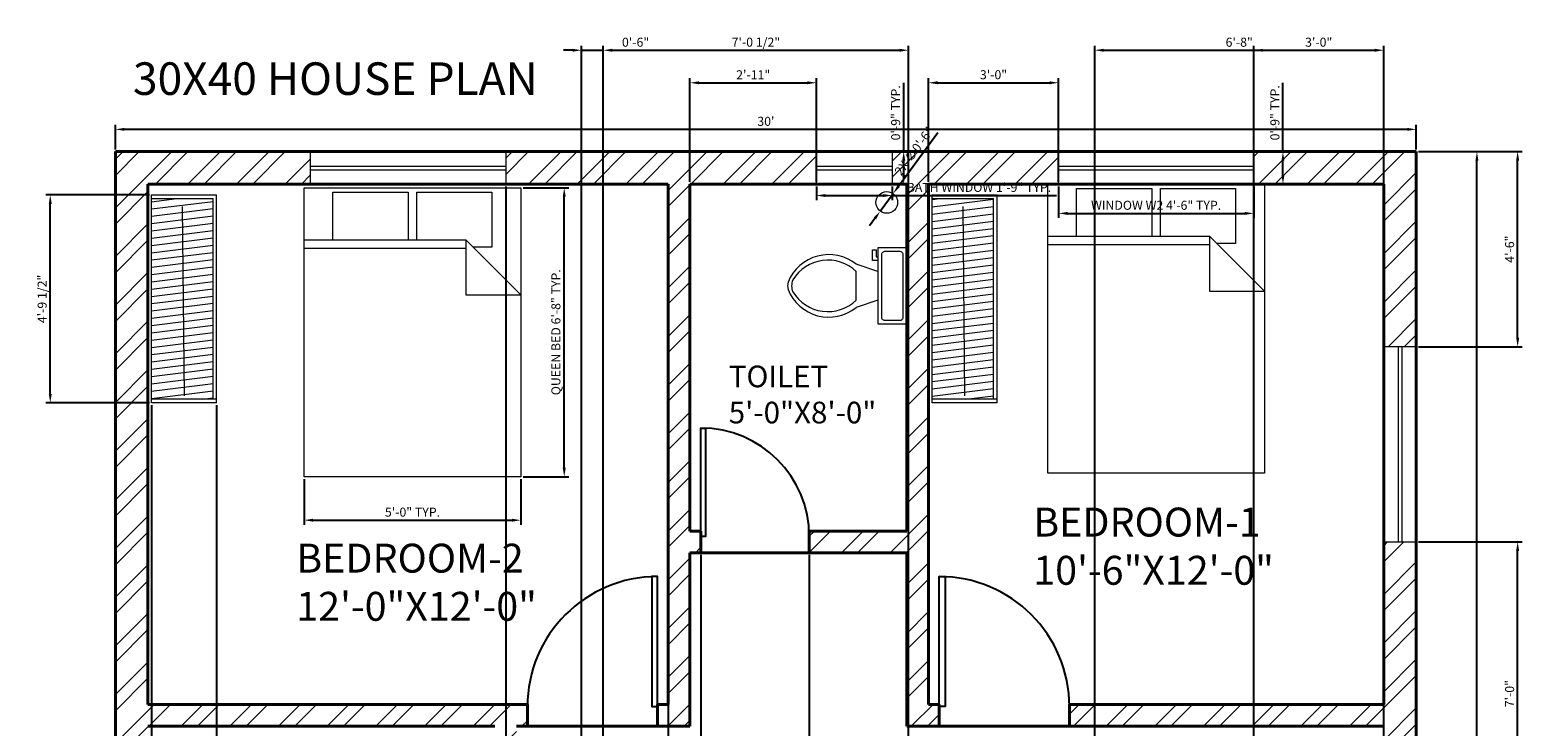
# Model space of a CAD drawing. Units: inches. Extents: x 201 to 622, y 55 to 632.
# Tile 3 of 3: x 209 to 622, y 439 to 632. Entities that reach past the tile are written whole.
import ezdxf

# ---------------------------------------------------------------- set-up
doc = ezdxf.new("R2010")
doc.units = ezdxf.units.IN
for name, color, linetype, lineweight in [('A-ANNO-DIMS', 2, 'Continuous', 18), ('A-ANNO-TITL', 7, 'Continuous', 25), ('A-AREA-IDEN', 7, 'Continuous', 18), ('A-DOOR', 4, 'Continuous', 25), ('A-FLOR-CASE', 8, 'Continuous', 18), ('A-FLOR-CASE-PATT', 8, 'Continuous', 13), ('A-FLOR-FIXT', 8, 'Continuous', 18), ('A-WALL', 7, 'Continuous', 40), ('A-WALL-PATT', 252, 'Continuous', 13)]:
    doc.layers.add(name, color=color, linetype=linetype, lineweight=lineweight)
doc.layers.add('A-FURN', color=152, linetype='Continuous', lineweight=18, true_color=0x2776bb)
doc.layers.add('A-GLAZ', color=152, linetype='Continuous', lineweight=18, true_color=0x2776bb)
doc.styles.get("Standard").update_dxf_attribs({"font": 'arial.ttf'})
doc.dimstyles.new('ISO-25', dxfattribs={"dimtxt": 2.5, "dimasz": 2.5, "dimexe": 1.25, "dimexo": 0.625, "dimtad": 1, "dimlunit": 3, "dimtxsty": 'Standard', "dimcen": 2.5, "dimadec": 0, "dimazin": 0, "dimtfac": 1, "dimtmove": 0, "dimatfit": 3, "dimfxl": 1, "dimarcsym": 0})

# ---------------------------------------------------------------- blocks, each defined once
blk = doc.blocks.new('*U2')
for p, q in [((0, 0), (0, -6)), ((-40, 0), (-40, -6))]:
    blk.add_line(p, q)
blk.add_lwpolyline([(0, 0), (0, 40), (-1.75, 40), (-1.75, 0)], close=True)
blk.add_arc((0, 0), 40, 90, 180)
blk = doc.blocks.new('*U3')
for p, q in [((0, 0), (0, -6)), ((40, 0), (40, -6))]:
    blk.add_line(p, q)
blk.add_lwpolyline([(0, 0), (0, 40), (1.75, 40), (1.75, 0)], close=True)
blk.add_arc((0, 0), 40, 0, 90)
blk = doc.blocks.new('Bed - Queen')
for p, q in [((0, -80.00003), (0, 0)), ((0, 0), (59.99999, 0)), ((59.99999, 0), (59.99999, -80.00003)), ((7.99999, -1.2), (28.79998, -1.2)), ((7.99999, -14.4), (7.99999, -1.2)), ((28.79998, -1.2), (28.79998, -14.4)), ((31.19999, -1.2), (51.99999, -1.2)), ((31.19999, -14.4), (31.19999, -1.2)), ((51.99999, -1.2), (51.99999, -16.4)), ((0, -14.4), (44.8, -14.4)), ((59.99999, -29.6), (44.8, -14.4)), ((44.8, -14.4), (44.8, -29.6)), ((51.99999, -16.4), (46.79936, -16.4)), ((44.8, -16.8), (0, -16.8)), ((44.8, -29.6), (59.99999, -29.6)), ((59.99999, -80.00003), (0, -80.00003))]:
    blk.add_line(p, q)
blk = doc.blocks.new('*U9')
for p, q in [((9.5, -6), (9.5, -2)), ((-8, -8.5), (-8, -8)), ((-7, -8), (-7, -9.5)), ((-4, -8), (-6, -14)), ((4, -8), (6, -14)), ((-10, -8.5), (-8, -8.5)), ((-10, -9.5), (-10, -8.5)), ((-7, -9.5), (-10, -9.5)), ((4, -14), (-4, -14))]:
    blk.add_line(p, q)
blk.add_lwpolyline([(10.5, -8), (10.5, 0), (-10.5, 0), (-10.5, -8)], close=True)
for points in [[(-9.5, -2), (-9.5, -6)], [(8.5, -1), (-8.5, -1)], [(-8.5, -7), (8.5, -7)]]:
    blk.add_lwpolyline(points)
for centre, radius, start, end in [((-8.62, -1.88), 0.884, 81.8699, 188.1301), ((8.62, -1.88), 0.884, 351.8699, 98.1301), ((-8.62, -6.12), 0.884, 171.8699, 278.1301), ((8.62, -6.12), 0.884, 261.8699, 8.1301), ((3.52, -21.58), 12.17, 141.4691, 247.9714), ((4.2, -21.82), 11.33, 136.3677, 238.9468), ((-3.52, -21.58), 12.17, 292.0284, 38.5307), ((-4.2, -21.82), 11.33, 301.053, 43.6321), ((0, -27.88), 4, 245.7318, 294.2682), ((0, -29), 4, 254.8605, 285.1395)]:
    blk.add_arc(centre, radius, start, end)
blk = doc.blocks.new('*D10')
at = {"layer": 'A-ANNO-DIMS', "color": 0, "lineweight": -2, "transparency": 16777216}
for p, q in [((592.99, 598.15), (610.4, 598.15)), ((609.15, 120.65), (609.15, 595.65)), ((592.99, 118.15), (610.4, 118.15))]:
    blk.add_line(p, q, dxfattribs=at)
at = {"layer": 'A-ANNO-DIMS', "color": 0, "transparency": 16777216}
for points in [[(608.73, 595.65), (609.56, 595.65), (609.15, 598.15)], [(608.73, 120.65), (609.56, 120.65), (609.15, 118.15)]]:
    blk.add_solid(points, dxfattribs=at)
at = {"layer": 'Defpoints', "color": 0, "transparency": 16777216}
for p in [(592.36, 598.15), (609.15, 598.15), (592.36, 118.15)]:
    blk.add_point(p, dxfattribs=at)
at = {"layer": 'A-ANNO-DIMS', "color": 0, "transparency": 16777216, "insert": (607.25, 358.15), "char_height": 2.5, "attachment_point": 5, "rotation": 90}
blk.add_mtext("40'", dxfattribs=at)
blk = doc.blocks.new('*D11')
at = {"layer": 'A-ANNO-DIMS', "color": 0, "lineweight": -2, "transparency": 16777216}
for p, q in [((232.36, 598.77), (232.36, 605.55)), ((589.86, 604.3), (234.86, 604.3)), ((592.36, 598.77), (592.36, 605.55))]:
    blk.add_line(p, q, dxfattribs=at)
at = {"layer": 'A-ANNO-DIMS', "color": 0, "transparency": 16777216}
for points in [[(234.86, 604.72), (234.86, 603.89), (232.36, 604.3)], [(589.86, 604.72), (589.86, 603.89), (592.36, 604.3)]]:
    blk.add_solid(points, dxfattribs=at)
at = {"layer": 'Defpoints', "color": 0, "transparency": 16777216}
for p in [(232.36, 604.3), (232.36, 598.15), (592.36, 598.15)]:
    blk.add_point(p, dxfattribs=at)
at = {"layer": 'A-ANNO-DIMS', "color": 0, "transparency": 16777216, "insert": (412.36, 606.2), "char_height": 2.5, "attachment_point": 5}
blk.add_mtext("30'", dxfattribs=at)
blk = doc.blocks.new('WIN-54')
for p, q in [((0, 5), (54, 5)), ((0, 4), (54, 4))]:
    blk.add_line(p, q)
blk.add_lwpolyline([(0, 9), (54, 9), (54, 0), (0, 0)], close=True)
blk = doc.blocks.new('WIN-21')
for p, q in [((0, 5), (21, 5)), ((0, 4), (21, 4))]:
    blk.add_line(p, q)
blk.add_lwpolyline([(0, 0), (0, 9), (21, 9), (21, 0)], close=True)
blk = doc.blocks.new('WIN-54-B')
for p, q in [((0, 5), (54, 5)), ((0, 4), (54, 4))]:
    blk.add_line(p, q)
blk.add_lwpolyline([(0, 9), (54, 9), (54, 0), (0, 0)], close=True)
blk = doc.blocks.new('*D17')
at = {"layer": 'A-ANNO-DIMS', "color": 0, "lineweight": -2, "transparency": 16777216}
for p, q in [((493.36, 588.52), (493.36, 579.8)), ((547.36, 588.52), (547.36, 579.8)), ((495.86, 581.05), (544.86, 581.05))]:
    blk.add_line(p, q, dxfattribs=at)
at = {"layer": 'A-ANNO-DIMS', "color": 0, "transparency": 16777216}
for points in [[(495.86, 581.46), (495.86, 580.63), (493.36, 581.05)], [(544.86, 581.46), (544.86, 580.63), (547.36, 581.05)]]:
    blk.add_solid(points, dxfattribs=at)
at = {"layer": 'Defpoints', "color": 0, "transparency": 16777216}
for p in [(493.36, 589.15), (547.36, 589.15), (547.36, 581.05)]:
    blk.add_point(p, dxfattribs=at)
at = {"layer": 'A-ANNO-DIMS', "color": 0, "transparency": 16777216, "insert": (520.36, 582.97), "char_height": 2.5, "attachment_point": 5}
blk.add_mtext('WINDOW W2 4\'-6" TYP.', dxfattribs=at)
blk = doc.blocks.new('*D18')
at = {"layer": 'A-ANNO-DIMS', "color": 0, "lineweight": -2, "transparency": 16777216}
for p, q in [((555.46, 598.15), (555.46, 617.14)), ((547.99, 598.15), (556.71, 598.15)), ((555.46, 591.65), (555.46, 595.65)), ((547.99, 589.15), (556.71, 589.15))]:
    blk.add_line(p, q, dxfattribs=at)
at = {"layer": 'A-ANNO-DIMS', "color": 0, "transparency": 16777216}
for points in [[(555.05, 595.65), (555.88, 595.65), (555.46, 598.15)], [(555.05, 591.65), (555.88, 591.65), (555.46, 589.15)]]:
    blk.add_solid(points, dxfattribs=at)
at = {"layer": 'Defpoints', "color": 0, "transparency": 16777216}
for p in [(547.36, 598.15), (555.46, 598.15), (547.36, 589.15)]:
    blk.add_point(p, dxfattribs=at)
at = {"layer": 'A-ANNO-DIMS', "color": 0, "transparency": 16777216, "insert": (553.56, 608.89), "char_height": 2.5, "attachment_point": 5, "rotation": 90}
blk.add_mtext('0\'-9" TYP.', dxfattribs=at)
blk = doc.blocks.new('*D19')
at = {"layer": 'A-ANNO-DIMS', "color": 0, "lineweight": -2, "transparency": 16777216}
for p, q in [((426.35, 588.52), (426.35, 584.75)), ((447.35, 588.52), (447.35, 584.75)), ((428.85, 586), (444.85, 586)), ((447.35, 586), (492.81, 586))]:
    blk.add_line(p, q, dxfattribs=at)
at = {"layer": 'A-ANNO-DIMS', "color": 0, "transparency": 16777216}
for points in [[(428.85, 586.41), (428.85, 585.58), (426.35, 586)], [(444.85, 586.41), (444.85, 585.58), (447.35, 586)]]:
    blk.add_solid(points, dxfattribs=at)
at = {"layer": 'Defpoints', "color": 0, "transparency": 16777216}
for p in [(426.35, 589.15), (447.35, 589.15), (447.35, 586)]:
    blk.add_point(p, dxfattribs=at)
at = {"layer": 'A-ANNO-DIMS', "color": 0, "transparency": 16777216, "insert": (471.33, 587.92), "char_height": 2.5, "attachment_point": 5}
blk.add_mtext('BATH WINDOW 1\'-9" TYP.', dxfattribs=at)
blk = doc.blocks.new('*D20')
at = {"layer": 'A-ANNO-DIMS', "color": 0, "lineweight": -2, "transparency": 16777216}
for p, q in [((450.5, 598.15), (450.5, 617.14)), ((447.98, 598.15), (451.75, 598.15)), ((450.5, 591.65), (450.5, 595.65)), ((447.98, 589.15), (451.75, 589.15))]:
    blk.add_line(p, q, dxfattribs=at)
at = {"layer": 'A-ANNO-DIMS', "color": 0, "transparency": 16777216}
for points in [[(450.09, 595.65), (450.92, 595.65), (450.5, 598.15)], [(450.09, 591.65), (450.92, 591.65), (450.5, 589.15)]]:
    blk.add_solid(points, dxfattribs=at)
at = {"layer": 'Defpoints', "color": 0, "transparency": 16777216}
for p in [(447.35, 598.15), (450.5, 598.15), (447.35, 589.15)]:
    blk.add_point(p, dxfattribs=at)
at = {"layer": 'A-ANNO-DIMS', "color": 0, "transparency": 16777216, "insert": (448.6, 608.89), "char_height": 2.5, "attachment_point": 5, "rotation": 90}
blk.add_mtext('0\'-9" TYP.', dxfattribs=at)
blk = doc.blocks.new('*D21')
at = {"layer": 'A-ANNO-DIMS', "color": 0, "lineweight": -2, "transparency": 16777216}
for p, q in [((345.19, 588.15), (357.81, 588.15)), ((356.56, 510.65), (356.56, 585.65)), ((345.19, 508.15), (357.81, 508.15))]:
    blk.add_line(p, q, dxfattribs=at)
at = {"layer": 'A-ANNO-DIMS', "color": 0, "transparency": 16777216}
for points in [[(356.15, 585.65), (356.98, 585.65), (356.56, 588.15)], [(356.15, 510.65), (356.98, 510.65), (356.56, 508.15)]]:
    blk.add_solid(points, dxfattribs=at)
at = {"layer": 'Defpoints', "color": 0, "transparency": 16777216}
for p in [(344.56, 588.15), (356.56, 588.15), (344.56, 508.15)]:
    blk.add_point(p, dxfattribs=at)
at = {"layer": 'A-ANNO-DIMS', "color": 0, "transparency": 16777216, "insert": (354.57, 548.15), "char_height": 2.5, "attachment_point": 5, "rotation": 90}
blk.add_mtext('QUEEN BED 6\'-8" TYP.', dxfattribs=at)
blk = doc.blocks.new('*D22')
at = {"layer": 'A-ANNO-DIMS', "color": 0, "lineweight": -2, "transparency": 16777216}
for p, q in [((284.56, 507.52), (284.56, 494.9)), ((344.56, 507.52), (344.56, 494.9)), ((287.06, 496.15), (342.06, 496.15))]:
    blk.add_line(p, q, dxfattribs=at)
at = {"layer": 'A-ANNO-DIMS', "color": 0, "transparency": 16777216}
for points in [[(287.06, 496.56), (287.06, 495.73), (284.56, 496.15)], [(342.06, 496.56), (342.06, 495.73), (344.56, 496.15)]]:
    blk.add_solid(points, dxfattribs=at)
at = {"layer": 'Defpoints', "color": 0, "transparency": 16777216}
for p in [(284.56, 508.15), (344.56, 508.15), (344.56, 496.15)]:
    blk.add_point(p, dxfattribs=at)
at = {"layer": 'A-ANNO-DIMS', "color": 0, "transparency": 16777216, "insert": (314.56, 498.05), "char_height": 2.5, "attachment_point": 5}
blk.add_mtext('5\'-0" TYP.', dxfattribs=at)
blk = doc.blocks.new('*D26')
at = {"layer": 'A-ANNO-DIMS', "color": 0, "lineweight": -2, "transparency": 16777216}
for p, q in [((547.36, 319.77), (547.36, 627.45)), ((549.86, 626.2), (580.86, 626.2)), ((583.36, 319.77), (583.36, 627.45))]:
    blk.add_line(p, q, dxfattribs=at)
at = {"layer": 'A-ANNO-DIMS', "color": 0, "transparency": 16777216}
for points in [[(549.86, 626.61), (549.86, 625.78), (547.36, 626.2)], [(580.86, 626.61), (580.86, 625.78), (583.36, 626.2)]]:
    blk.add_solid(points, dxfattribs=at)
at = {"layer": 'Defpoints', "color": 0, "transparency": 16777216}
for p in [(583.36, 626.2), (547.36, 319.15), (583.36, 319.15)]:
    blk.add_point(p, dxfattribs=at)
at = {"layer": 'A-ANNO-DIMS', "color": 0, "transparency": 16777216, "insert": (565.36, 628.1), "char_height": 2.5, "attachment_point": 5}
blk.add_mtext('3\'-0"', dxfattribs=at)
blk = doc.blocks.new('*D27')
at = {"layer": 'A-ANNO-DIMS', "color": 0, "lineweight": -2, "transparency": 16777216}
for p, q in [((358.86, 626.2), (356.36, 626.2)), ((361.36, 289.77), (361.36, 627.45)), ((361.36, 626.2), (367.36, 626.2)), ((367.36, 289.77), (367.36, 627.45)), ((369.86, 626.2), (380.26, 626.2))]:
    blk.add_line(p, q, dxfattribs=at)
at = {"layer": 'A-ANNO-DIMS', "color": 0, "transparency": 16777216}
for points in [[(358.86, 626.61), (358.86, 625.78), (361.36, 626.2)], [(369.86, 626.61), (369.86, 625.78), (367.36, 626.2)]]:
    blk.add_solid(points, dxfattribs=at)
at = {"layer": 'Defpoints', "color": 0, "transparency": 16777216}
for p in [(367.36, 626.2), (361.36, 289.15), (367.36, 289.15)]:
    blk.add_point(p, dxfattribs=at)
at = {"layer": 'A-ANNO-DIMS', "color": 0, "transparency": 16777216, "insert": (376.31, 628.1), "char_height": 2.5, "attachment_point": 5}
blk.add_mtext('0\'-6"', dxfattribs=at)
blk = doc.blocks.new('*D29')
at = {"layer": 'A-ANNO-DIMS', "color": 0, "lineweight": -2, "transparency": 16777216}
for p, q in [((340.36, 588.52), (340.36, 55.85)), ((385.36, 588.52), (385.36, 55.85)), ((342.86, 57.1), (382.86, 57.1))]:
    blk.add_line(p, q, dxfattribs=at)
at = {"layer": 'A-ANNO-DIMS', "color": 0, "transparency": 16777216}
for points in [[(342.86, 57.51), (342.86, 56.68), (340.36, 57.1)], [(382.86, 57.51), (382.86, 56.68), (385.36, 57.1)]]:
    blk.add_solid(points, dxfattribs=at)
at = {"layer": 'Defpoints', "color": 0, "transparency": 16777216}
for p in [(340.36, 589.15), (385.36, 589.15), (385.36, 57.1)]:
    blk.add_point(p, dxfattribs=at)
at = {"layer": 'A-ANNO-DIMS', "color": 0, "transparency": 16777216, "insert": (362.86, 59), "char_height": 2.5, "attachment_point": 5}
blk.add_mtext('3\'-9"', dxfattribs=at)
blk = doc.blocks.new('*D30')
at = {"layer": 'A-ANNO-DIMS', "color": 0, "lineweight": -2, "transparency": 16777216}
for p, q in [((391.36, 589.77), (391.36, 618.45)), ((393.86, 617.2), (423.85, 617.2)), ((426.35, 589.77), (426.35, 618.45))]:
    blk.add_line(p, q, dxfattribs=at)
at = {"layer": 'A-ANNO-DIMS', "color": 0, "transparency": 16777216}
for points in [[(393.86, 617.61), (393.86, 616.78), (391.36, 617.2)], [(423.85, 617.61), (423.85, 616.78), (426.35, 617.2)]]:
    blk.add_solid(points, dxfattribs=at)
at = {"layer": 'Defpoints', "color": 0, "transparency": 16777216}
for p in [(426.35, 617.2), (391.36, 589.15), (426.35, 589.15)]:
    blk.add_point(p, dxfattribs=at)
at = {"layer": 'A-ANNO-DIMS', "color": 0, "transparency": 16777216, "insert": (408.86, 619.08), "char_height": 2.5, "attachment_point": 5}
blk.add_mtext('2\'-11"', dxfattribs=at)
blk = doc.blocks.new('*D31')
at = {"layer": 'A-ANNO-DIMS', "color": 0, "lineweight": -2, "transparency": 16777216}
for p, q in [((457.36, 589.77), (457.36, 618.45)), ((459.86, 617.2), (490.86, 617.2)), ((493.36, 589.77), (493.36, 618.45))]:
    blk.add_line(p, q, dxfattribs=at)
at = {"layer": 'A-ANNO-DIMS', "color": 0, "transparency": 16777216}
for points in [[(459.86, 617.61), (459.86, 616.78), (457.36, 617.2)], [(490.86, 617.61), (490.86, 616.78), (493.36, 617.2)]]:
    blk.add_solid(points, dxfattribs=at)
at = {"layer": 'Defpoints', "color": 0, "transparency": 16777216}
for p in [(493.36, 617.2), (457.36, 589.15), (493.36, 589.15)]:
    blk.add_point(p, dxfattribs=at)
at = {"layer": 'A-ANNO-DIMS', "color": 0, "transparency": 16777216, "insert": (475.36, 619.1), "char_height": 2.5, "attachment_point": 5}
blk.add_mtext('3\'-0"', dxfattribs=at)
blk = doc.blocks.new('*D32')
at = {"layer": 'A-ANNO-DIMS', "color": 0, "lineweight": -2, "transparency": 16777216}
for p, q in [((592.99, 598.15), (621.66, 598.15)), ((620.41, 546.65), (620.41, 595.65)), ((592.99, 544.15), (621.66, 544.15))]:
    blk.add_line(p, q, dxfattribs=at)
at = {"layer": 'A-ANNO-DIMS', "color": 0, "transparency": 16777216}
for points in [[(620, 595.65), (620.83, 595.65), (620.41, 598.15)], [(620, 546.65), (620.83, 546.65), (620.41, 544.15)]]:
    blk.add_solid(points, dxfattribs=at)
at = {"layer": 'Defpoints', "color": 0, "transparency": 16777216}
for p in [(592.36, 598.15), (620.41, 598.15), (592.36, 544.15)]:
    blk.add_point(p, dxfattribs=at)
at = {"layer": 'A-ANNO-DIMS', "color": 0, "transparency": 16777216, "insert": (618.51, 571.15), "char_height": 2.5, "attachment_point": 5, "rotation": 90}
blk.add_mtext('4\'-6"', dxfattribs=at)
blk = doc.blocks.new('*D33')
at = {"layer": 'A-ANNO-DIMS', "color": 0, "lineweight": -2, "transparency": 16777216}
for p, q in [((592.99, 490.15), (621.66, 490.15)), ((620.41, 408.65), (620.41, 487.65)), ((592.99, 406.15), (621.66, 406.15))]:
    blk.add_line(p, q, dxfattribs=at)
at = {"layer": 'A-ANNO-DIMS', "color": 0, "transparency": 16777216}
for points in [[(620, 487.65), (620.83, 487.65), (620.41, 490.15)], [(620, 408.65), (620.83, 408.65), (620.41, 406.15)]]:
    blk.add_solid(points, dxfattribs=at)
at = {"layer": 'Defpoints', "color": 0, "transparency": 16777216}
for p in [(592.36, 490.15), (620.41, 490.15), (592.36, 406.15)]:
    blk.add_point(p, dxfattribs=at)
at = {"layer": 'A-ANNO-DIMS', "color": 0, "transparency": 16777216, "insert": (618.51, 448.15), "char_height": 2.5, "attachment_point": 5, "rotation": 90}
blk.add_mtext('7\'-0"', dxfattribs=at)
blk = doc.blocks.new('*D40')
at = {"layer": 'A-ANNO-DIMS', "color": 0, "lineweight": -2, "transparency": 16777216}
for p, q in [((394.36, 486.52), (394.36, 55.85)), ((424.36, 486.52), (424.36, 55.85)), ((396.86, 57.1), (421.86, 57.1))]:
    blk.add_line(p, q, dxfattribs=at)
at = {"layer": 'A-ANNO-DIMS', "color": 0, "transparency": 16777216}
for points in [[(396.86, 57.51), (396.86, 56.68), (394.36, 57.1)], [(421.86, 57.51), (421.86, 56.68), (424.36, 57.1)]]:
    blk.add_solid(points, dxfattribs=at)
at = {"layer": 'Defpoints', "color": 0, "transparency": 16777216}
for p in [(394.36, 487.15), (424.36, 487.15), (424.36, 57.1)]:
    blk.add_point(p, dxfattribs=at)
at = {"layer": 'A-ANNO-DIMS', "color": 0, "transparency": 16777216, "insert": (409.36, 59), "char_height": 2.5, "attachment_point": 5}
blk.add_mtext('2\'-6"', dxfattribs=at)
blk = doc.blocks.new('*D48')
at = {"layer": 'A-ANNO-DIMS', "color": 0, "lineweight": -2, "transparency": 16777216}
for p, q in [((367.36, 118.77), (367.36, 627.45)), ((369.86, 626.2), (449.36, 626.2)), ((451.86, 118.77), (451.86, 627.45))]:
    blk.add_line(p, q, dxfattribs=at)
at = {"layer": 'A-ANNO-DIMS', "color": 0, "transparency": 16777216}
for points in [[(369.86, 626.61), (369.86, 625.78), (367.36, 626.2)], [(449.36, 626.61), (449.36, 625.78), (451.86, 626.2)]]:
    blk.add_solid(points, dxfattribs=at)
at = {"layer": 'Defpoints', "color": 0, "transparency": 16777216}
for p in [(451.86, 626.2), (367.36, 118.15), (451.86, 118.15)]:
    blk.add_point(p, dxfattribs=at)
at = {"layer": 'A-ANNO-DIMS', "color": 0, "transparency": 16777216, "insert": (409.61, 628.11), "char_height": 2.5, "attachment_point": 5}
blk.add_mtext('7\'-0 1/2"', dxfattribs=at)
blk = doc.blocks.new('*D55')
at = {"layer": 'A-ANNO-DIMS', "color": 0, "lineweight": -2, "transparency": 16777216}
for p, q in [((503.36, 403.77), (503.36, 627.45)), ((505.86, 626.2), (580.86, 626.2)), ((583.36, 403.77), (583.36, 627.45))]:
    blk.add_line(p, q, dxfattribs=at)
at = {"layer": 'A-ANNO-DIMS', "color": 0, "transparency": 16777216}
for points in [[(505.86, 626.61), (505.86, 625.78), (503.36, 626.2)], [(580.86, 626.61), (580.86, 625.78), (583.36, 626.2)]]:
    blk.add_solid(points, dxfattribs=at)
at = {"layer": 'Defpoints', "color": 0, "transparency": 16777216}
for p in [(583.36, 626.2), (503.36, 403.15), (583.36, 403.15)]:
    blk.add_point(p, dxfattribs=at)
at = {"layer": 'A-ANNO-DIMS', "color": 0, "transparency": 16777216, "insert": (543.36, 628.1), "char_height": 2.5, "attachment_point": 5}
blk.add_mtext('6\'-8"', dxfattribs=at)
blk = doc.blocks.new('*D56')
at = {"layer": 'A-ANNO-DIMS', "color": 0, "lineweight": -2, "transparency": 16777216}
for p, q in [((242.36, 527.98), (242.36, 55.85)), ((260.36, 527.98), (260.36, 55.85)), ((244.86, 57.1), (257.86, 57.1))]:
    blk.add_line(p, q, dxfattribs=at)
at = {"layer": 'A-ANNO-DIMS', "color": 0, "transparency": 16777216}
for points in [[(244.86, 57.51), (244.86, 56.68), (242.36, 57.1)], [(257.86, 57.51), (257.86, 56.68), (260.36, 57.1)]]:
    blk.add_solid(points, dxfattribs=at)
at = {"layer": 'Defpoints', "color": 0, "transparency": 16777216}
for p in [(242.36, 528.6), (260.36, 528.6), (260.36, 57.1)]:
    blk.add_point(p, dxfattribs=at)
at = {"layer": 'A-ANNO-DIMS', "color": 0, "transparency": 16777216, "insert": (251.36, 59), "char_height": 2.5, "attachment_point": 5}
blk.add_mtext('1\'-6"', dxfattribs=at)
blk = doc.blocks.new('*D57')
at = {"layer": 'A-ANNO-DIMS', "color": 0, "lineweight": -2, "transparency": 16777216}
for p, q in [((241.74, 586.15), (213.06, 586.15)), ((214.31, 531.1), (214.31, 583.65)), ((241.74, 528.6), (213.06, 528.6))]:
    blk.add_line(p, q, dxfattribs=at)
at = {"layer": 'A-ANNO-DIMS', "color": 0, "transparency": 16777216}
for points in [[(213.9, 583.65), (214.73, 583.65), (214.31, 586.15)], [(213.9, 531.1), (214.73, 531.1), (214.31, 528.6)]]:
    blk.add_solid(points, dxfattribs=at)
at = {"layer": 'Defpoints', "color": 0, "transparency": 16777216}
for p in [(214.31, 586.15), (242.36, 586.15), (242.36, 528.6)]:
    blk.add_point(p, dxfattribs=at)
at = {"layer": 'A-ANNO-DIMS', "color": 0, "transparency": 16777216, "insert": (212.39, 557.38), "char_height": 2.5, "attachment_point": 5, "rotation": 90}
blk.add_mtext('4\'-9 1/2"', dxfattribs=at)
blk = doc.blocks.new('*D59')
at = {"layer": 'A-ANNO-DIMS', "color": 0, "lineweight": -2, "transparency": 16777216}
for p, q in [((459.95, 603.36), (449.06, 588.53)), ((444.03, 581.68), (447.58, 586.51)), ((442.56, 579.66), (441.08, 577.64))]:
    blk.add_line(p, q, dxfattribs=at)
at = {"layer": 'A-ANNO-DIMS', "color": 0, "transparency": 16777216}
for points in [[(448.73, 588.78), (449.4, 588.28), (447.58, 586.51)], [(442.22, 579.91), (442.89, 579.41), (444.03, 581.68)]]:
    blk.add_solid(points, dxfattribs=at)
at = {"layer": 'Defpoints', "color": 0, "transparency": 16777216}
for p in [(447.58, 586.51), (444.03, 581.68)]:
    blk.add_point(p, dxfattribs=at)
at = {"layer": 'A-ANNO-DIMS', "color": 0, "transparency": 16777216, "insert": (453.66, 598.12), "char_height": 2.5, "attachment_point": 5, "rotation": 53.7299}
blk.add_mtext('2X ∅0\'-6"', dxfattribs=at)

msp = doc.modelspace()

# ---------------------------------------------------------------- hatches: boundary and pattern name
at = {"layer": 'A-FLOR-CASE-PATT'}
h = msp.add_hatch(dxfattribs=at)
h.set_pattern_fill('ANSI31', color=256, scale=0.629921, angle=-37.9287, style=0)
h.paths.add_polyline_path([(242.362, 529.603), (259.362, 529.603), (259.362, 585.147), (242.362, 585.147)])
h = msp.add_hatch(dxfattribs=at)
h.set_pattern_fill('ANSI31', color=256, scale=0.629921, angle=-37.9287, style=0)
h.paths.add_polyline_path([(458.362, 529.603), (475.362, 529.603), (475.362, 585.147), (458.362, 585.147)])
at = {"layer": 'A-WALL-PATT'}
h = msp.add_hatch(dxfattribs=at)
h.set_pattern_fill('ANSI32', color=256)
h.paths.add_polyline_path([(241.362, 589.147), (286.362, 589.147), (286.362, 598.147), (232.362, 598.147), (232.362, 418.002), (241.362, 418.002), (241.362, 439.147), (337.362, 439.147), (337.362, 436.147), (343.362, 436.147), (343.362, 439.147), (346.362, 439.147), (346.362, 445.147), (241.362, 445.147)])
h.paths.add_polyline_path([(394.362, 493.147), (391.362, 493.147), (391.362, 589.147), (426.354, 589.147), (426.354, 598.147), (340.362, 598.147), (340.362, 589.147), (385.362, 589.147), (385.362, 445.147), (382.362, 445.147), (382.362, 439.147), (391.362, 439.147), (391.362, 487.147), (394.362, 487.147)])
h.paths.add_polyline_path([(457.362, 589.147), (493.362, 589.147), (493.362, 598.147), (447.354, 598.147), (447.354, 589.147), (451.362, 589.147), (451.362, 493.147), (424.362, 493.147), (424.362, 487.147), (451.362, 487.147), (451.362, 439.147), (460.362, 439.147), (460.362, 445.147), (457.362, 445.147)])
h.paths.add_polyline_path([(592.362, 598.147), (547.362, 598.147), (547.362, 589.147), (550.362, 589.147), (583.362, 589.147), (583.362, 544.147), (592.362, 544.147)])
h.paths.add_polyline_path([(592.362, 490.147), (583.362, 490.147), (583.362, 445.147), (496.362, 445.147), (496.362, 439.147), (583.362, 439.147), (583.362, 406.147), (592.362, 406.147)])
h.paths.add_polyline_path([(592.362, 352.147), (583.362, 352.147), (583.362, 319.147), (532.362, 319.147), (532.362, 313.147), (583.362, 313.147), (583.362, 256.147), (592.362, 256.147)])
h.paths.add_polyline_path([(592.362, 202.147), (583.362, 202.147), (583.362, 145.147), (549.11, 145.147), (549.11, 136.147), (592.362, 136.147)])
h.paths.add_polyline_path([(493.362, 313.147), (496.362, 313.147), (496.362, 319.147), (487.362, 319.147), (487.362, 259.147), (409.362, 259.147), (409.362, 250.147), (415.362, 250.147), (415.362, 253.147), (469.362, 253.147), (469.362, 187.147), (448.415, 187.147), (448.415, 178.147), (451.858, 178.147), (451.858, 175.147), (457.858, 175.147), (457.858, 178.147), (475.362, 178.147), (475.362, 253.147), (493.362, 253.147)])
h.paths.add_polyline_path([(495.11, 145.147), (457.858, 145.147), (451.858, 145.147), (451.858, 136.147), (495.11, 136.147)])
h.paths.add_polyline_path([(367.362, 178.147), (370.362, 178.147), (370.362, 183.547), (370.362, 187.147), (367.362, 187.147), (367.362, 220.147), (361.362, 220.147), (361.362, 127.147), (326.862, 127.147), (326.862, 118.147), (367.362, 118.147)])
h.paths.add_polyline_path([(272.862, 127.147), (241.362, 127.147), (241.362, 259.147), (361.362, 259.147), (361.362, 256.147), (361.962, 256.147), (367.362, 256.147), (367.362, 289.147), (361.362, 289.147), (361.362, 265.147), (241.362, 265.147), (241.362, 385.147), (361.362, 385.147), (361.362, 361.147), (367.362, 361.147), (367.362, 391.147), (343.362, 391.147), (343.362, 406.147), (338.862, 406.147), (337.362, 406.147), (337.362, 391.147), (241.362, 391.147), (241.362, 397.002), (232.362, 397.002), (232.362, 118.147), (272.862, 118.147)])
h.paths.add_polyline_path([(417.381, 187.147), (415.362, 187.147), (415.362, 220.147), (410.862, 220.147), (409.362, 220.147), (409.362, 187.147), (406.181, 187.147, -0.0250471), (406.362, 183.547), (406.362, 178.147), (417.381, 178.147)])

# ---------------------------------------------------------------- linework, layer by layer
at = {"layer": 'A-FLOR-CASE'}
for p, q in [((242.362, 586.147), (260.362, 586.147)), ((242.362, 528.603), (242.362, 586.147)), ((242.362, 585.147), (259.362, 585.147)), ((250.862, 582.938), (251.34, 530.599)), ((259.362, 529.603), (259.362, 585.147)), ((260.362, 528.603), (260.362, 586.147)), ((458.362, 586.147), (476.362, 586.147)), ((458.362, 528.603), (458.362, 586.147)), ((458.362, 585.147), (475.362, 585.147)), ((466.862, 582.938), (467.34, 530.599)), ((475.362, 529.603), (475.362, 585.147)), ((476.362, 528.603), (476.362, 586.147)), ((260.362, 529.603), (242.362, 529.603)), ((476.362, 529.603), (458.362, 529.603)), ((260.362, 528.603), (242.362, 528.603)), ((476.362, 528.603), (458.362, 528.603))]:
    msp.add_line(p, q, dxfattribs=at)
at = {"layer": 'A-FLOR-FIXT'}
msp.add_circle((445.81, 584.095), 3, dxfattribs=at)
at = {"layer": 'A-WALL'}
for p, q in [((232.362, 598.147), (592.362, 598.147)), ((232.362, 118.147), (232.362, 598.147)), ((592.362, 598.147), (592.362, 118.147)), ((241.362, 589.147), (385.362, 589.147)), ((241.362, 445.147), (241.362, 589.147)), ((385.362, 445.147), (385.362, 589.147)), ((391.362, 589.147), (451.362, 589.147)), ((391.362, 493.147), (391.362, 589.147)), ((451.362, 493.147), (451.362, 589.147)), ((457.362, 445.147), (457.362, 589.147)), ((457.362, 589.147), (583.362, 589.147)), ((583.362, 589.147), (583.362, 445.147)), ((391.362, 493.147), (394.362, 493.147)), ((394.362, 487.147), (394.362, 493.147)), ((424.362, 487.147), (424.362, 493.147)), ((424.362, 493.147), (451.362, 493.147)), ((391.362, 439.147), (391.362, 487.147)), ((391.362, 487.147), (451.362, 487.147)), ((451.362, 439.147), (451.362, 487.147)), ((241.362, 445.147), (346.362, 445.147)), ((346.362, 445.147), (346.362, 439.147)), ((382.362, 445.147), (382.362, 439.147)), ((382.362, 445.147), (385.362, 445.147)), ((457.362, 445.147), (460.362, 445.147)), ((460.362, 445.147), (460.362, 439.147)), ((496.362, 445.147), (496.362, 439.147)), ((496.362, 445.147), (583.362, 445.147)), ((241.362, 439.147), (337.362, 439.147)), ((343.362, 439.147), (391.362, 439.147)), ((451.362, 439.147), (583.362, 439.147))]:
    msp.add_line(p, q, dxfattribs=at)

# ---------------------------------------------------------------- block references
at = {"layer": 'A-DOOR'}
for name, p, xscale, yscale, zscale in [('*U3', (394.362, 491.647), 0.75, 0.75, 0.75), ('*U2', (382.362, 444.547), 0.9, 0.9, 0.9), ('*U3', (460.362, 444.547), 0.9, 0.9, 0.9)]:
    msp.add_blockref(name, p, dxfattribs=dict(at, xscale=xscale, yscale=yscale, zscale=zscale))
at = {"layer": 'A-FLOR-FIXT', "rotation": 270}
msp.add_blockref('*U9', (451.362, 560.99), dxfattribs=at)
at = {"layer": 'A-FURN'}
for p in [(284.562, 588.147), (490.362, 589.147)]:
    msp.add_blockref('Bed - Queen', p, dxfattribs=at)
at = {"layer": 'A-GLAZ'}
for name, p in [('WIN-54', (286.362, 589.147)), ('WIN-21', (426.354, 589.147)), ('WIN-54-B', (493.362, 589.147))]:
    msp.add_blockref(name, p, dxfattribs=at)
at = {"layer": 'A-GLAZ', "extrusion": (0, 0, -1), "zscale": -1, "rotation": 270}
msp.add_blockref('WIN-54', (-592.362, 544.147), dxfattribs=at)

# ---------------------------------------------------------------- texts
at = {"layer": 'A-ANNO-TITL', "insert": (237.199, 622.845), "char_height": 9, "attachment_point": 1}
msp.add_mtext_dynamic_manual_height_columns('30X40 HOUSE PLAN', width=123.9439, gutter_width=12.5, heights=[0], dxfattribs=at)
at = {"layer": 'A-AREA-IDEN', "attachment_point": 1}
for s, width, insert, char_height in [('TOILET\\P5\'-0"X8\'-0"', 38.71373, (402.079, 538.931), 6), ('BEDROOM-1\\P10\'-6"X12\'-0"', 68.77314, (486.363, 499.619), 8), ('BEDROOM-2\\P12\'-0"X12\'-0"', 68.77314, (282.394, 489.643), 8)]:
    msp.add_mtext_dynamic_manual_height_columns(s, width=width, gutter_width=12.5, heights=[0], dxfattribs=dict(at, insert=insert, char_height=char_height))

# ---------------------------------------------------------------- dimensions: what is measured, and where the dimension line sits
at = {"layer": 'A-ANNO-DIMS'}
for base, p1, p2, override, picture, middle in [((367.362, 626.197), (361.362, 289.147), (367.362, 289.147), {"dimdec": 1, "dimlfac": 1, "dimrnd": 0, "dimzin": 1, "dimdsep": 46, "dimlunit": 4, "dimfrac": 2}, '*D27', (376.31, 628.099)), ((451.858, 626.197), (367.362, 118.147), (451.858, 118.147), {"dimdec": 1, "dimlfac": 1, "dimrnd": 0, "dimzin": 1, "dimdsep": 46, "dimlunit": 4, "dimfrac": 2}, '*D48', (409.61, 628.115)), ((583.362, 626.197), (503.362, 403.147), (583.362, 403.147), {"dimdec": 1, "dimlfac": 1, "dimrnd": 0, "dimzin": 1, "dimdsep": 46, "dimlunit": 4, "dimfrac": 2}, '*D55', (543.362, 628.099)), ((583.362, 626.197), (547.362, 319.147), (583.362, 319.147), {"dimdec": 1, "dimlfac": 1, "dimrnd": 0, "dimzin": 1, "dimdsep": 46, "dimlunit": 4, "dimfrac": 2}, '*D26', (565.362, 628.1)), ((232.362, 604.302), (592.362, 598.147), (232.362, 598.147), {"dimclrd": 0, "dimclre": 0, "dimclrt": 0}, '*D11', (412.362, 606.204)), ((385.362, 57.097), (340.362, 589.147), (385.362, 589.147), {"dimdec": 1, "dimlfac": 1, "dimrnd": 0, "dimzin": 1, "dimdsep": 46, "dimlunit": 4, "dimfrac": 2}, '*D29', (362.862, 59)), ((260.362, 57.097), (242.362, 528.603), (260.362, 528.603), {"dimdec": 1, "dimlfac": 1, "dimrnd": 0, "dimzin": 1, "dimdsep": 46, "dimlunit": 4, "dimfrac": 2}, '*D56', (251.362, 58.999)), ((424.362, 57.097), (394.362, 487.147), (424.362, 487.147), {"dimdec": 1, "dimlfac": 1, "dimrnd": 0, "dimzin": 1, "dimdsep": 46, "dimlunit": 4, "dimfrac": 2}, '*D40', (409.362, 58.999))]:
    dim = msp.add_linear_dim(base=base, p1=p1, p2=p2, dimstyle='ISO-25', override=override, dxfattribs=at)
    dim.commit()
    dim.dimension.update_dxf_attribs({"geometry": picture, "text_midpoint": middle})
for base, p1, p2, angle, override, picture, middle in [((426.354, 617.197), (391.362, 589.147), (426.354, 589.147), 0, {"dimdec": 1, "dimlfac": 1, "dimrnd": 0, "dimzin": 1, "dimdsep": 46, "dimlunit": 4, "dimfrac": 2}, '*D30', (408.858, 619.077)), ((493.362, 617.197), (457.362, 589.147), (493.362, 589.147), 0, {"dimdec": 1, "dimlfac": 1, "dimrnd": 0, "dimzin": 1, "dimdsep": 46, "dimlunit": 4, "dimfrac": 2}, '*D31', (475.362, 619.1)), ((609.147, 598.147), (592.362, 118.147), (592.362, 598.147), 90, {"dimclrd": 0, "dimclre": 0, "dimclrt": 0}, '*D10', (607.246, 358.147)), ((620.412, 598.147), (592.362, 544.147), (592.362, 598.147), 90, {"dimdec": 1, "dimlfac": 1, "dimrnd": 0, "dimzin": 1, "dimdsep": 46, "dimlunit": 4, "dimfrac": 2}, '*D32', (618.51, 571.147)), ((214.312, 586.147), (242.362, 528.603), (242.362, 586.147), 90, {"dimdec": 1, "dimlfac": 1, "dimrnd": 0, "dimzin": 1, "dimdsep": 46, "dimlunit": 4, "dimfrac": 2}, '*D57', (212.394, 557.375)), ((620.412, 490.147), (592.362, 406.147), (592.362, 490.147), 90, {"dimdec": 1, "dimlfac": 1, "dimrnd": 0, "dimzin": 1, "dimdsep": 46, "dimlunit": 4, "dimfrac": 2}, '*D33', (618.51, 448.147))]:
    dim = msp.add_linear_dim(base=base, p1=p1, p2=p2, angle=angle, dimstyle='ISO-25', override=override, dxfattribs=at)
    dim.commit()
    dim.dimension.update_dxf_attribs({"geometry": picture, "text_midpoint": middle})
for base, p1, p2, text, picture, middle in [((450.504, 598.147), (447.354, 589.147), (447.354, 598.147), '<> TYP.', '*D20', (448.603, 608.892)), ((555.462, 598.147), (547.362, 589.147), (547.362, 598.147), '<> TYP.', '*D18', (553.56, 608.892)), ((356.562, 588.147), (344.562, 508.147), (344.562, 588.147), 'QUEEN BED <> TYP.', '*D21', (354.567, 548.147))]:
    dim = msp.add_linear_dim(base=base, p1=p1, p2=p2, angle=90, text=text, dimstyle='ISO-25', override={"dimdec": 1, "dimlfac": 1, "dimrnd": 0, "dimzin": 1, "dimdsep": 46, "dimlunit": 4, "dimfrac": 2}, dxfattribs=at)
    dim.commit()
    dim.dimension.update_dxf_attribs({"geometry": picture, "text_midpoint": middle})
dim = msp.add_diameter_dim_2p(p1=(444.035, 581.676), p2=(447.584, 586.514), text='2X <>', dimstyle='ISO-25', override={"dimdec": 1, "dimlfac": 1, "dimrnd": 0, "dimzin": 1, "dimdsep": 46, "dimlunit": 4, "dimfrac": 2}, dxfattribs=at)
dim.commit()
dim.dimension.update_dxf_attribs({"geometry": '*D59', "text_midpoint": (455.245, 596.953), "dimtype": 163})
for base, p1, p2, text, picture, middle in [((447.354, 585.997), (426.354, 589.147), (447.354, 589.147), 'BATH WINDOW <> TYP.', '*D19', (471.333, 587.916)), ((547.362, 581.047), (493.362, 589.147), (547.362, 589.147), 'WINDOW W2 <> TYP.', '*D17', (520.362, 582.966)), ((344.562, 496.147), (284.562, 508.147), (344.562, 508.147), '<> TYP.', '*D22', (314.562, 498.049))]:
    dim = msp.add_linear_dim(base=base, p1=p1, p2=p2, text=text, dimstyle='ISO-25', override={"dimdec": 1, "dimlfac": 1, "dimrnd": 0, "dimzin": 1, "dimdsep": 46, "dimlunit": 4, "dimfrac": 2}, dxfattribs=at)
    dim.commit()
    dim.dimension.update_dxf_attribs({"geometry": picture, "text_midpoint": middle})

doc.saveas('drawing.dxf')
